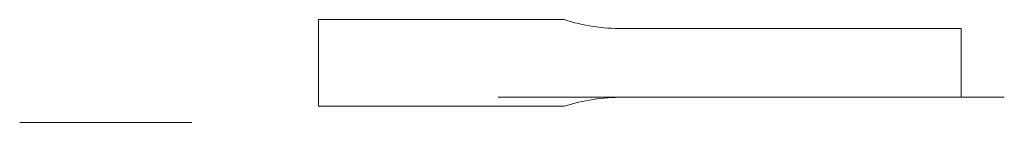
# Model space of a CAD drawing. Units: millimetres. Extents: x 678 to 1079, y 68 to 110.
import ezdxf

# ---------------------------------------------------------------- set-up
doc = ezdxf.new("R2010")
doc.units = ezdxf.units.MM
doc.layers.add('M-CONS', color=8, linetype='Continuous', lineweight=18)

msp = doc.modelspace()

# ---------------------------------------------------------------- linework, layer by layer
at = {"layer": 'M-CONS'}
msp.add_lwpolyline([(1061.12, 106.19), (923.23, 106.19, -0.077158), (899.58, 109.86), (799.58, 109.86), (799.58, 74.52), (899.58, 74.52, -0.077158), (923.23, 78.19), (1061.12, 78.19)], format="xyb", close=True, dxfattribs=at)
at = {"layer": 'M-CONS', "extrusion": (0, -1, 0), "elevation": -78.19}
msp.add_lwpolyline([(1030.72, 18.5), (880.72, 18.5, 1), (880.72, 2.5), (1030.72, 2.5, 1)], format="xyb", close=True, dxfattribs=at)
at = {"layer": 'M-CONS', "extrusion": (0, -1, 0)}
for centre, radius in [((1061.12, 10.5, -78.19), 17.5), ((1061.12, 10.5, -78.19), 12), ((712.96, 12.99, -67.95), 35), ((712.96, 12.99, -67.95), 26)]:
    msp.add_circle(centre, radius, dxfattribs=at)

doc.saveas('drawing.dxf')
